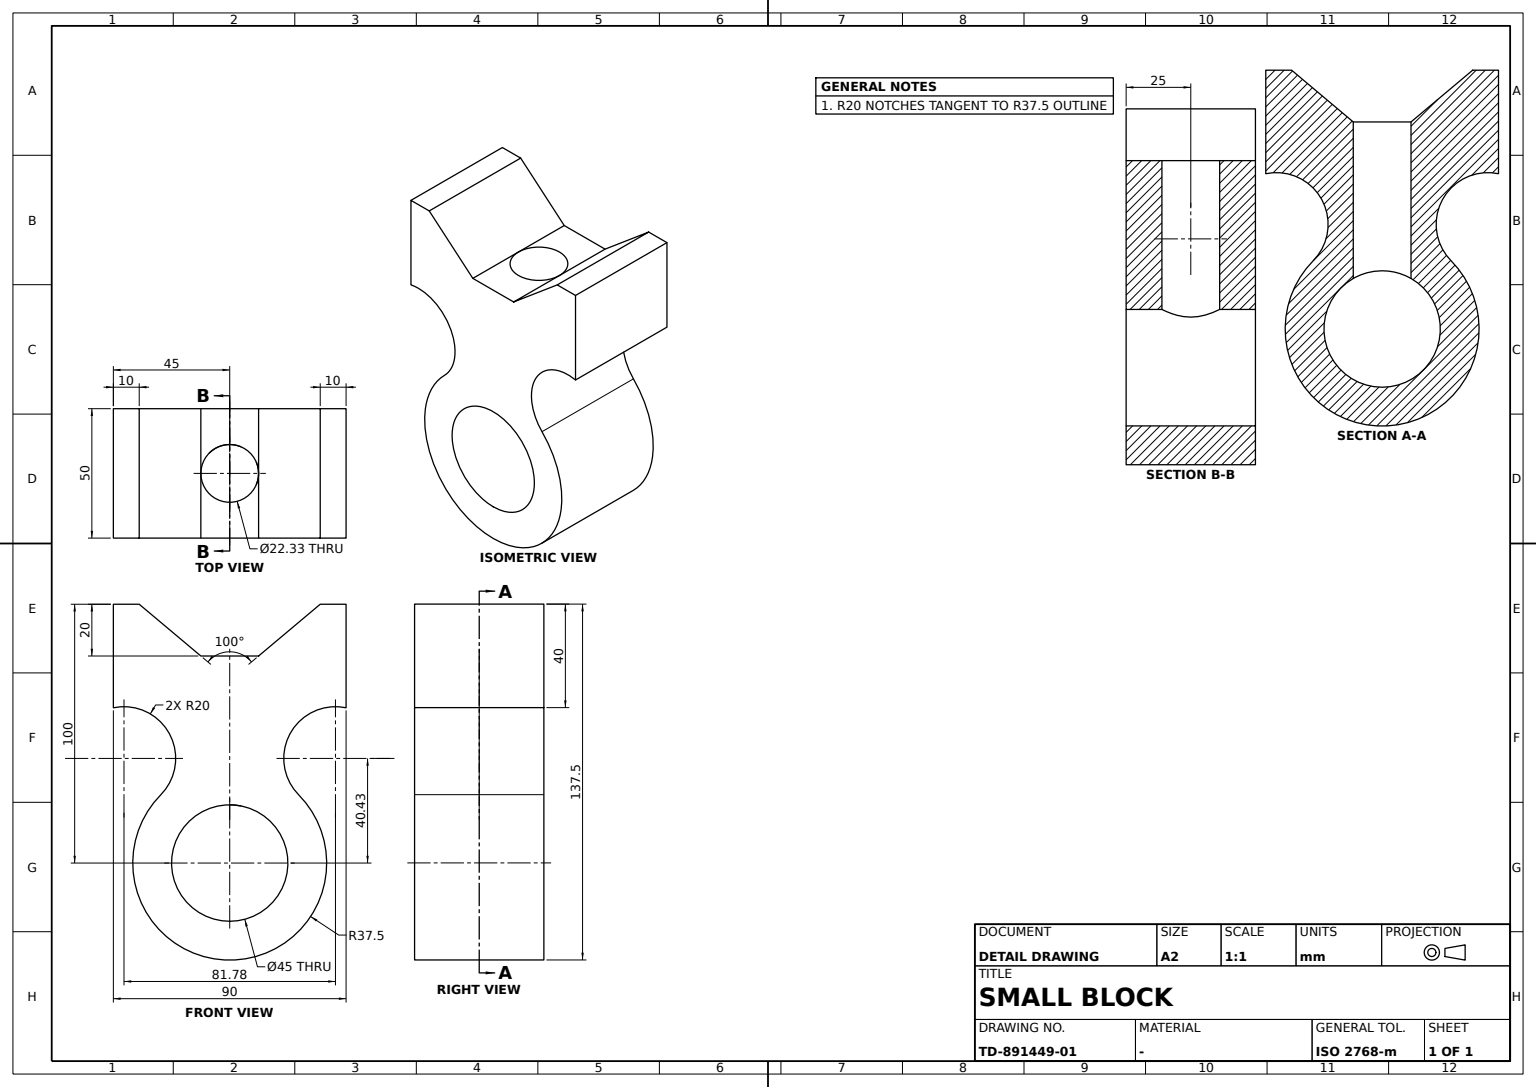
CATIA V5 part; units mm, degrees
sketch "Sketch1" plane through (0, 0, 0) normal (1, 0, 0) x (0, 1, 0)
  arc A0 (-26.6667, 26.3655) -> (26.6667, 26.3655) centre (0, 0) ccw
  circle A1 centre (0, 0) radius 22.5
  line L0 (-45, 60) -> (-45, 100)
  line L1 (-45, 100) -> (-35, 100)
  line L2 (-35, 100) -> (-11.1649, 80)
  line L3 (-11.1649, 80) -> (11.1649, 80)
  line L4 (11.1649, 80) -> (35, 100)
  point P0 (35, 100)
  line L5 (35, 100) -> (45, 100)
  line L6 (45, 100) -> (45, 60)
  point P1 (-17.9589, 32.92)
  arc A2 (45, 60) -> (26.6667, 26.3655) centre (40.8889, 40.4271) ccw
  point P2 (26.6667, 26.3655)
  arc A3 (-45, 60) -> (-26.6667, 26.3655) centre (-40.8889, 40.4271) cw
  point P3 (-26.6667, 26.3655)
  dimension "angle L2 L4" = 100
  dimension "distance L3 L1" = 20
  dimension "length L1" = 10
  dimension "distance L0 L6" = 90
  dimension "length L6" = 40
  dimension "radius A1" = 22.5
  dimension "radius A0" = 37.5
  dimension "length L0" = 40
  dimension "radius A2" = 20
  dimension "radius A3" = 20
  dimension "distance L5 x axis" = 100
  constraint vertical L0 y-axis
  constraint vertical L6 y-axis
  constraint horizontal L1 x-axis
  constraint horizontal L3 x-axis
  constraint horizontal L5 x-axis
  constraint coincidence P0 L1
  constraint coincidence P1 A0
  constraint coincidence A2 P2
  constraint coincidence P2 A0
  constraint coincidence A3 P3
  constraint coincidence P3 A0
  constraint symmetry L6 L0 y-axis
  constraint symmetry L4 L2 y-axis
  constraint tangency A2 A0
  constraint tangency A0 A3
extrude "Pad1" add sketch "Sketch1" along normal mid plane 50
sketch "Sketch2" plane through (0, 0, 80) normal (0, 0, 1) x (1, 0, 0)
  circle A0 centre (0, 0) radius 11.1649
  point P0 (0, -11.1649)
  line L0 (-25, -11.1649) -> (25, -11.1649) construction
  constraint coincidence A0 P0
  constraint coincidence P0 y-axis
  constraint tangency A0 L0
extrude "Pocket1" cut sketch "Sketch2" against normal up to next
